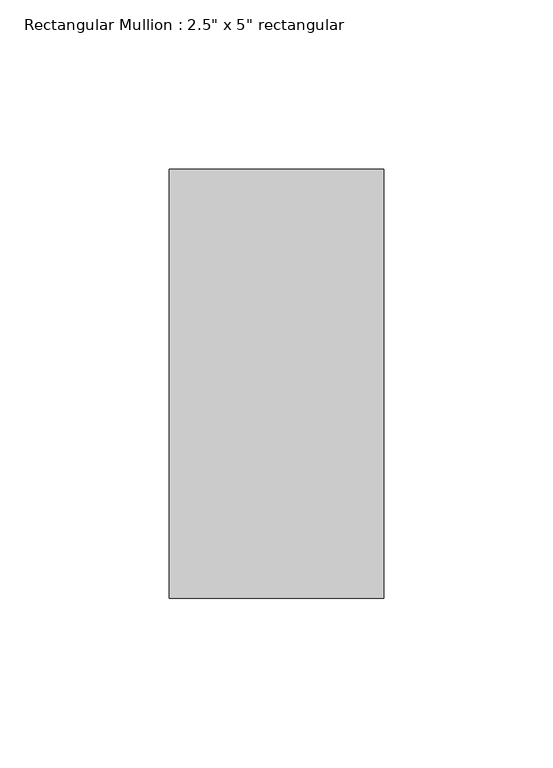
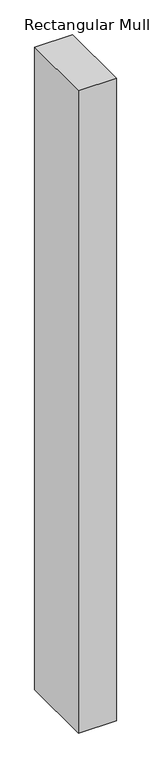
"""IFC4 building model written with IfcOpenShell, lengths in millimetres: member geometry."""

from ifc_helpers import new_model, si_unit, frame, origin, place, context, project, spatial, polyline, outline, extrude, source, transform, mapped, element, save


def member_af5dd0cd(model_context):
    return source(origin(), model_context, "Body", "SweptSolid", [
        extrude(outline(polyline([(0.0, 63.5), (0.0, -63.5), (-63.5, -63.5), (-63.5, 63.5), (0.0, 63.5)])), frame((0.0, 0.0, -1137.3648635), z_axis=(0.0, 0.0, 1.0), x_axis=(1.0, 0.0, 0.0)), (0.0, 0.0, 1.0), 1137.3648635),
    ])


if __name__ == "__main__":
    model = new_model("IFC4")
    model_context = context("Model", 3, world=origin())
    ifc_project = project(units=[si_unit("LENGTHUNIT", "METRE", prefix="MILLI")], contexts=[model_context])
    site = spatial("IfcSite", under=ifc_project)
    building = spatial("IfcBuilding", under=site)
    placement = place(None, origin())
    member_shape = member_af5dd0cd(model_context)
    element("IfcMember", 1, ObjectType="Rectangular Mullion : 2.5\" x 5\" rectangular", at=placement, inside=building, context=model_context, shape_type="MappedRepresentation", body=[
        mapped(member_shape, transform((0.0, 0.0, 0.0), x_axis=(1.0, 0.0, 0.0), y_axis=(0.0, 1.0, 0.0), z_axis=(0.0, 0.0, 1.0))),
    ])
    save(model, "model.ifc")

# Revit data of these elements
# Type "Rectangular Mullion : 2.5\" x 5\" rectangular"
#   built-in parameter 1007304 = 0.416667 (stored number, unit not read)
#   built-in parameter 1007301 = 0.104167 (stored number, unit not read)
#   built-in parameter 1007300 = 0.104167 (stored number, unit not read)
# Element 1 (IfcMember, "Rectangular Mullion : 2.5\" x 5\" rectangular")
#   Materials on its faces: "Aluminum"
# Materials
#   "Aluminum": class "Metal", colour RGB 247 247 247, transparency 0, Description = "Aluminum 6061", Cost = 0
